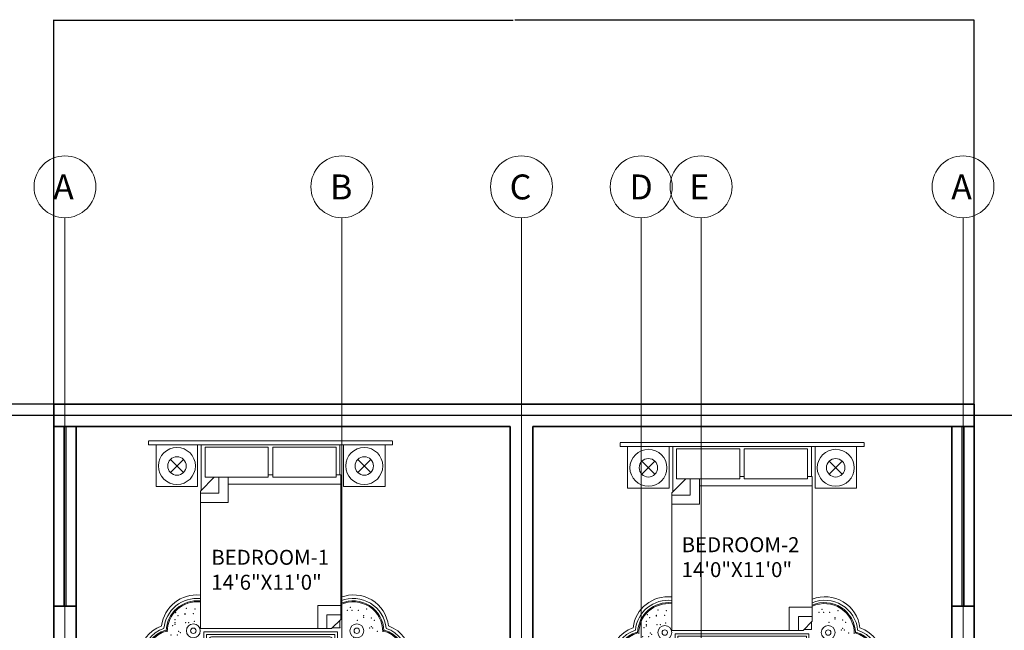
# Model space of a CAD drawing. Units: inches. Extents: x 5716 to 6907, y 12769 to 13594.
# Tile 16 of 17: x 6254 to 6648, y 13349 to 13594. Entities that reach past the tile are written whole.
import ezdxf

# ---------------------------------------------------------------- set-up
doc = ezdxf.new("R2010")
doc.units = ezdxf.units.IN
for name, color, linetype, lineweight in [('A-ANNO-DIMS', 2, 'Continuous', 18), ('A-AREA-IDEN', 7, 'Continuous', 18), ('A-FURN', 8, 'Continuous', 18), ('A-GLAZ', 4, 'Continuous', 18), ('A-GRID', 8, 'Continuous', 13), ('A-GRID-IDEN', 7, 'Continuous', 18), ('A-WALL', 7, 'Continuous', 35)]:
    doc.layers.add(name, color=color, linetype=linetype, lineweight=lineweight)
doc.styles.get("Standard").update_dxf_attribs({"font": 'arial.ttf'})
doc.dimstyles.get("Standard").update_dxf_attribs({"dimtxt": 0.18, "dimasz": 0.18, "dimexe": 0.18, "dimexo": 0.0625, "dimgap": 0.09, "dimtad": 0, "dimtih": 1, "dimtoh": 1, "dimdec": 4, "dimzin": 0, "dimdsep": 46, "dimtxsty": 'Standard', "dimcen": 0.09, "dimadec": 0, "dimazin": 0, "dimtfac": 1, "dimtdec": 4, "dimtofl": 0, "dimtmove": 0, "dimatfit": 3, "dimfxl": 1, "dimtolj": 1, "dimtzin": 0, "dimarcsym": 0})

# ---------------------------------------------------------------- blocks, each defined once
blk = doc.blocks.new('A$C1EC128A1')
for p, q in [((0.115, 3.56), (3.019, 3.56)), ((0.115, 3.555), (0.115, 3.511)), ((3.019, 3.555), (3.019, 3.511)), ((0.115, 3.511), (3.019, 3.511)), ((0.203, 3.511), (0.203, 3.462)), ((0.203, 3.46), (0.203, 3.016)), ((0.698, 3.511), (0.698, 3.016)), ((0.742, 3.511), (0.742, 2.972)), ((0.786, 3.484), (1.539, 3.484)), ((0.786, 3.484), (0.786, 3.126)), ((1.539, 3.126), (1.539, 3.484)), ((1.594, 3.126), (1.594, 3.484)), ((1.594, 3.484), (2.348, 3.484)), ((2.348, 3.484), (2.348, 3.126)), ((2.392, 3.511), (2.392, 3.154)), ((2.436, 3.511), (2.436, 3.016)), ((2.931, 3.511), (2.931, 3.016)), ((0.374, 3.181), (0.53, 3.337)), ((0.374, 3.337), (0.53, 3.181)), ((2.604, 3.337), (2.759, 3.181)), ((2.759, 3.337), (2.604, 3.181)), ((0.731, 2.961), (0.896, 3.126)), ((0.786, 3.126), (1.539, 3.126)), ((0.951, 3.126), (0.951, 2.934)), ((1.061, 3.126), (1.061, 2.824)), ((1.539, 3.154), (1.594, 3.154)), ((1.594, 3.126), (2.348, 3.126)), ((2.348, 3.154), (2.403, 3.154)), ((2.403, 3.154), (2.403, 1.432)), ((0.203, 3.016), (0.698, 3.016)), ((0.731, 2.961), (0.731, 1.322)), ((0.731, 2.934), (0.951, 2.934)), ((1.061, 3.044), (2.403, 3.044)), ((2.931, 3.016), (2.436, 3.016)), ((0.731, 2.824), (1.061, 2.824)), ((2.128, 1.597), (2.403, 1.597)), ((2.128, 1.597), (2.128, 1.322)), ((2.238, 1.487), (2.238, 1.322)), ((2.238, 1.487), (2.403, 1.487)), ((2.293, 1.322), (2.403, 1.432)), ((2.392, 1.421), (2.392, 1.333)), ((0.731, 1.322), (2.293, 1.322)), ((2.304, 1.333), (2.392, 1.333)), ((0.772, 1.282), (2.363, 1.282)), ((0.772, 0.939), (0.772, 1.282)), ((0.802, 1.252), (2.333, 1.252)), ((0.802, 0.969), (0.802, 1.252)), ((0.832, 1.029), (0.832, 1.192)), ((0.862, 1.222), (2.273, 1.222)), ((2.303, 1.192), (2.303, 1.029)), ((2.333, 1.252), (2.333, 0.969)), ((2.363, 1.282), (2.363, 0.939)), ((2.363, 0.939), (0.772, 0.939)), ((2.333, 0.969), (0.802, 0.969)), ((2.273, 0.999), (0.862, 0.999))]:
    blk.add_line(p, q)
for centre, radius in [((0.452, 3.259), 0.22), ((2.682, 3.259), 0.22), ((0.452, 3.259), 0.11), ((2.682, 3.259), 0.11), ((0.647, 1.296), 0.0826), ((0.647, 1.296), 0.0326), ((2.593, 1.296), 0.0826), ((2.593, 1.296), 0.0326), ((0.418, 0.972), 0.0826), ((0.418, 0.972), 0.0326), ((2.822, 0.972), 0.0826), ((2.822, 0.972), 0.0326), ((0.647, 0.647), 0.0826), ((2.593, 0.647), 0.0826), ((0.647, 0.647), 0.0326), ((2.593, 0.647), 0.0326), ((1.111, 0.374), 0.0826), ((1.111, 0.374), 0.0326), ((1.613, 0.323), 0.0826), ((1.613, 0.323), 0.0326), ((2.129, 0.374), 0.0826), ((2.129, 0.374), 0.0326)]:
    blk.add_circle(centre, radius)
for centre, radius, start, end in [((0.685, 1.305), 0.418, 83.7824, 173.2515), ((0.688, 1.288), 0.393, 83.8157, 174.53), ((0.692, 1.284), 0.369, 83.9971, 177.9976), ((2.555, 1.305), 0.418, 6.7485, 111.2795), ((2.552, 1.288), 0.393, 5.47, 112.249), ((2.548, 1.284), 0.369, 2.0024, 113.1536), ((0.691, 1.287), 0.354, 83.6051, 180.6699), ((2.549, 1.287), 0.354, 359.3301, 114.3551), ((0.405, 0.972), 0.405, 109.4527, 180), ((0.412, 0.972), 0.371, 108.0256, 180), ((0.411, 0.972), 0.343, 105.7891, 180), ((0.412, 0.972), 0.331, 104.766, 180), ((2.828, 0.972), 0.331, 0, 75.234), ((2.829, 0.972), 0.343, 0, 74.2109), ((2.828, 0.972), 0.371, 0, 71.9744), ((2.835, 0.972), 0.405, 0, 70.5473), ((0.862, 1.192), 0.03, 90, 180), ((2.273, 1.192), 0.03, 0, 90), ((2.008, 0.994), 0.365, 1.1782, 13.4812), ((0.405, 0.972), 0.405, 180, 250.5473), ((0.412, 0.972), 0.371, 180, 251.9744), ((0.411, 0.972), 0.343, 180, 254.2109), ((0.412, 0.972), 0.331, 180, 255.234), ((0.862, 1.029), 0.03, 180, 270), ((1.217, 0.977), 0.365, 186.0197, 214.7326), ((1.217, 0.977), 0.265, 188.3055, 214.7326), ((1.62, 0.972), 0.319, 185.9507, 354.0493), ((1.62, 0.972), 0.305, 186.2151, 353.7849), ((1.62, 0.972), 0.121, 195.7695, 344.2305), ((1.62, 0.972), 0.105, 198.3291, 341.6709), ((2.008, 0.994), 0.265, 327.6239, 348.1186), ((2.273, 1.029), 0.03, 270, 0), ((2.008, 0.994), 0.365, 327.6239, 1.1782), ((2.828, 0.972), 0.331, 284.766, 0), ((2.829, 0.972), 0.343, 285.7891, 0), ((2.828, 0.972), 0.371, 288.0256, 0), ((2.835, 0.972), 0.405, 289.4527, 0), ((1.403, 1.107), 0.492, 214.7326, 239.1926), ((1.817, 1.115), 0.492, 303.1639, 327.6239), ((1.403, 1.107), 0.592, 214.7326, 239.1926), ((1.817, 1.115), 0.592, 303.1639, 327.6239), ((0.685, 0.639), 0.418, 186.7485, 287.3233), ((0.688, 0.656), 0.393, 185.47, 288.0175), ((0.692, 0.66), 0.369, 182.0024, 288.623), ((0.691, 0.657), 0.354, 179.3301, 289.5945), ((1.524, 1.309), 0.828, 239.1926, 256.6746), ((1.524, 1.309), 0.728, 239.1926, 256.6746), ((1.599, 1.627), 1.054, 256.6746, 271.1782), ((1.599, 1.627), 1.054, 271.1782, 285.6819), ((1.688, 1.312), 0.728, 285.6819, 303.1639), ((1.688, 1.312), 0.828, 285.6819, 303.1639), ((2.549, 0.657), 0.354, 250.4055, 0.6699), ((2.548, 0.66), 0.369, 251.377, 357.9976), ((2.552, 0.656), 0.393, 251.9825, 354.53), ((2.555, 0.639), 0.418, 252.6767, 353.2515), ((1.599, 1.627), 1.154, 256.6746, 271.1782), ((1.599, 1.627), 1.154, 271.1782, 285.6819), ((1.133, 0.498), 0.367, 208.2914, 306.3479), ((1.133, 0.484), 0.367, 208.2914, 306.3479), ((1.133, 0.461), 0.369, 208.9302, 306.0262), ((1.132, 0.42), 0.369, 209.2201, 306.079), ((2.107, 0.498), 0.367, 233.6521, 331.7086), ((2.107, 0.484), 0.367, 233.6521, 331.7086), ((2.107, 0.461), 0.369, 233.9738, 331.0698), ((2.108, 0.42), 0.369, 233.921, 330.7799), ((1.614, 0.43), 0.349, 220.6393, 270.9052), ((1.614, 0.416), 0.349, 220.6393, 270.9052), ((1.62, 0.4), 0.36, 221.3878, 270), ((1.62, 0.36), 0.36, 221.4185, 270), ((1.626, 0.43), 0.349, 269.0948, 319.3607), ((1.626, 0.416), 0.349, 269.0948, 319.3607), ((1.62, 0.4), 0.36, 270, 318.6122), ((1.62, 0.36), 0.36, 270, 318.5815)]:
    blk.add_arc(centre, radius, start, end)
for p in [(0.565, 1.565), (0.666, 1.556), (2.482, 1.538), (2.518, 1.574), (2.537, 1.538), (2.61, 1.538), (2.71, 1.556), (0.428, 1.428), (0.438, 1.51), (0.465, 1.474), (0.547, 1.501), (0.547, 1.492), (0.647, 1.501), (0.657, 1.41), (2.601, 1.419), (2.674, 1.474), (2.674, 1.456), (2.765, 1.447), (2.801, 1.419), (0.401, 1.355), (0.428, 1.392), (0.428, 1.373), (0.474, 1.291), (0.556, 1.392), (0.593, 1.392), (2.392, 1.333), (2.747, 1.328), (2.765, 1.346), (2.783, 1.328), (2.838, 1.291), (0.319, 1.182), (0.383, 1.246), (0.456, 1.246), (0.474, 1.182), (0.492, 1.273), (0.556, 1.172), (2.555, 1.218), (0.118, 1.109), (0.182, 1.145), (0.209, 1.099), (0.237, 1.072), (0.246, 1.063), (0.301, 1.118), (0.456, 1.127), (0.657, 1.118), (2.455, 1.136), (2.482, 1.063), (2.646, 1.063), (2.774, 1.163), (2.893, 1.109), (2.966, 1.145), (3.057, 1.099), (0.118, 0.981), (0.155, 1.026), (0.182, 1.017), (0.182, 0.944), (0.593, 1.045), (0.684, 0.962), (1.303, 0.939), (1.317, 0.939), (2.473, 1.026), (2.537, 1.035), (2.573, 1.035), (2.601, 0.962), (2.966, 1.035), (0.173, 0.917), (0.182, 0.898), (0.209, 0.871), (0.474, 0.835), (0.602, 0.835), (0.666, 0.853), (0.693, 0.862), (0.812, 0.835), (0.999, 0.826), (1.067, 0.853), (1.076, 0.835), (1.113, 0.825), (1.186, 0.853), (1.259, 0.871), (1.277, 0.844), (2.026, 0.825), (2.044, 0.844), (2.044, 0.844), (2.153, 0.926), (2.153, 0.844), (2.591, 0.871), (2.984, 0.825), (3.002, 0.889), (3.002, 0.825), (3.102, 0.926), (0.173, 0.798), (0.255, 0.78), (0.264, 0.789), (0.301, 0.752), (0.511, 0.78), (0.784, 0.734), (0.803, 0.734), (1.067, 0.816), (1.113, 0.798), (1.159, 0.78), (1.159, 0.761), (1.204, 0.761), (1.25, 0.752), (1.259, 0.761), (1.259, 0.743), (1.259, 0.734), (1.277, 0.743), (1.305, 0.752), (1.314, 0.771), (1.323, 0.816), (1.898, 0.707), (1.907, 0.807), (1.907, 0.752), (2.062, 0.798), (2.381, 0.752), (2.409, 0.716), (2.418, 0.78), (2.537, 0.816), (2.591, 0.78), (2.756, 0.78), (2.829, 0.716), (2.847, 0.707), (2.883, 0.798), (0.31, 0.67), (0.401, 0.606), (0.41, 0.661), (0.447, 0.588), (0.465, 0.615), (0.492, 0.661), (0.821, 0.698), (0.903, 0.67), (0.912, 0.652), (0.949, 0.588), (1.152, 0.684), (1.152, 0.684), (1.152, 0.684), (1.286, 0.688), (1.323, 0.698), (1.323, 0.67), (1.35, 0.698), (1.35, 0.679), (1.356, 0.601), (1.359, 0.688), (1.451, 0.643), (1.487, 0.679), (1.578, 0.624), (1.651, 0.661), (1.651, 0.661), (1.779, 0.661), (1.88, 0.679), (1.88, 0.661), (1.884, 0.612), (2.007, 0.679), (2.086, 0.703), (2.263, 0.597), (2.381, 0.634), (2.4, 0.624), (2.737, 0.661), (0.465, 0.533), (0.501, 0.506), (0.529, 0.478), (0.593, 0.524), (0.73, 0.478), (0.73, 0.469), (0.757, 0.497), (0.812, 0.524), (0.83, 0.57), (0.867, 0.542), (0.967, 0.533), (0.976, 0.515), (1.031, 0.515), (1.333, 0.504), (1.898, 0.469), (2.19, 0.561), (2.263, 0.533), (2.272, 0.533), (2.409, 0.515), (2.455, 0.478), (2.482, 0.478), (2.61, 0.478), (2.646, 0.469), (2.747, 0.551), (2.756, 0.515), (2.81, 0.551), (0.465, 0.451), (0.538, 0.387), (0.556, 0.451), (0.574, 0.387), (0.602, 0.442), (0.62, 0.46), (0.638, 0.424), (0.739, 0.405), (0.739, 0.405), (0.912, 0.414), (0.921, 0.36), (0.93, 0.442), (0.985, 0.405), (1.341, 0.36), (1.396, 0.369), (1.414, 0.396), (1.642, 0.369), (1.77, 0.405), (1.852, 0.405), (2.144, 0.442), (2.245, 0.433), (2.29, 0.387), (2.601, 0.46), (0.638, 0.35), (0.693, 0.332), (0.81, 0.282), (0.985, 0.323), (1.086, 0.241), (1.204, 0.323), (1.213, 0.25), (1.332, 0.296), (1.341, 0.296), (1.35, 0.296), (1.378, 0.341), (1.496, 0.35), (1.651, 0.259), (1.852, 0.268), (1.87, 0.277), (1.916, 0.35), (2.327, 0.323), (2.43, 0.324), (0.985, 0.149), (1.131, 0.159), (1.35, 0.203), (1.451, 0.204), (1.487, 0.204), (1.606, 0.149), (1.67, 0.204), (1.724, 0.186), (1.962, 0.195), (2.08, 0.204), (2.135, 0.213), (2.217, 0.177)]:
    blk.add_point(p)
blk = doc.blocks.new('WIN-GLAZING-72IN')
for p, q in [((0, 0), (0, -72)), ((1, 0), (1, -72))]:
    blk.add_line(p, q)
blk = doc.blocks.new('*D49')
at = {"layer": 'A-ANNO-DIMS', "color": 0, "lineweight": -2, "transparency": 16777216}
for p, q in [((6267.41, 13440.21), (6267.41, 13594.38)), ((6267.59, 13594.2), (6451.62, 13594.2)), ((6636.23, 13594.2), (6452.2, 13594.2)), ((6636.41, 13440.21), (6636.41, 13594.38))]:
    blk.add_line(p, q, dxfattribs=at)
at = {"layer": 'A-ANNO-DIMS', "color": 0, "transparency": 16777216}
for points in [[(6267.59, 13594.23), (6267.59, 13594.17), (6267.41, 13594.2)], [(6636.23, 13594.23), (6636.23, 13594.17), (6636.41, 13594.2)]]:
    blk.add_solid(points, dxfattribs=at)
at = {"layer": 'Defpoints', "color": 0, "transparency": 16777216}
for p in [(6636.41, 13594.2), (6267.41, 13440.15), (6636.41, 13440.15)]:
    blk.add_point(p, dxfattribs=at)
at = {"layer": 'A-ANNO-DIMS', "color": 0, "transparency": 16777216, "insert": (6451.91, 13594.2), "char_height": 0.18, "attachment_point": 5}
blk.add_mtext('\\A1;369', dxfattribs=at)
blk = doc.blocks.new('*D52')
at = {"layer": 'A-ANNO-DIMS', "color": 0, "lineweight": -2, "transparency": 16777216}
for p, q in [((6267.34, 13440.15), (5716.04, 13440.15)), ((5716.22, 13439.97), (5716.22, 13140.83)), ((5716.22, 12841.33), (5716.22, 13140.47)), ((6267.34, 12841.15), (5716.04, 12841.15))]:
    blk.add_line(p, q, dxfattribs=at)
at = {"layer": 'A-ANNO-DIMS', "color": 0, "transparency": 16777216}
for points in [[(5716.19, 13439.97), (5716.25, 13439.97), (5716.22, 13440.15)], [(5716.19, 12841.33), (5716.25, 12841.33), (5716.22, 12841.15)]]:
    blk.add_solid(points, dxfattribs=at)
at = {"layer": 'Defpoints', "color": 0, "transparency": 16777216}
for p in [(6267.41, 13440.15), (5716.22, 12841.15), (6267.41, 12841.15)]:
    blk.add_point(p, dxfattribs=at)
at = {"layer": 'A-ANNO-DIMS', "color": 0, "transparency": 16777216, "insert": (5716.22, 13140.65), "char_height": 0.18, "attachment_point": 5}
blk.add_mtext('\\A1;599', dxfattribs=at)
blk = doc.blocks.new('*D58')
at = {"layer": 'A-ANNO-DIMS', "color": 0, "lineweight": -2, "transparency": 16777216}
for p, q in [((6736.67, 13435.65), (5716.04, 13435.65)), ((5716.22, 13435.47), (5716.22, 13365.33)), ((5716.22, 13294.83), (5716.22, 13364.97)), ((6736.67, 13294.65), (5716.04, 13294.65))]:
    blk.add_line(p, q, dxfattribs=at)
at = {"layer": 'A-ANNO-DIMS', "color": 0, "transparency": 16777216}
for points in [[(5716.19, 13435.47), (5716.25, 13435.47), (5716.22, 13435.65)], [(5716.19, 13294.83), (5716.25, 13294.83), (5716.22, 13294.65)]]:
    blk.add_solid(points, dxfattribs=at)
at = {"layer": 'Defpoints', "color": 0, "transparency": 16777216}
for p in [(6736.73, 13435.65), (5716.22, 13294.65), (6736.73, 13294.65)]:
    blk.add_point(p, dxfattribs=at)
at = {"layer": 'A-ANNO-DIMS', "color": 0, "transparency": 16777216, "insert": (5716.22, 13365.15), "char_height": 0.18, "attachment_point": 5}
blk.add_mtext('\\A1;141', dxfattribs=at)

msp = doc.modelspace()

# ---------------------------------------------------------------- linework, layer by layer
at = {"layer": 'A-GRID'}
for p, q in [((6271.91, 12841.15), (6271.91, 13514.96)), ((6382.91, 12841.15), (6382.91, 13514.96)), ((6454.91, 12841.15), (6454.91, 13514.96)), ((6502.91, 12841.15), (6502.91, 13514.96)), ((6526.91, 12841.15), (6526.91, 13514.96)), ((6631.91, 12841.15), (6631.91, 13514.96)), ((6267.41, 13435.65), (6736.73, 13435.65))]:
    msp.add_line(p, q, dxfattribs=at)
at = {"layer": 'A-GRID-IDEN'}
for centre in [(6271.91, 13527.35), (6382.91, 13527.35), (6454.91, 13527.35), (6502.91, 13527.35), (6526.91, 13527.35), (6631.91, 13527.35)]:
    msp.add_circle(centre, 12.4, dxfattribs=at)
at = {"layer": 'A-WALL'}
for p, q in [((6267.41, 13440.15), (6267.41, 12841.15)), ((6267.41, 13440.15), (6636.41, 13440.15)), ((6636.41, 13440.15), (6636.41, 13185.15)), ((6267.41, 13431.15), (6450.41, 13431.15)), ((6276.41, 13431.15), (6276.41, 13299.15)), ((6450.41, 13431.15), (6450.41, 13290.15)), ((6459.41, 13431.15), (6459.41, 13290.15)), ((6459.41, 13431.15), (6636.41, 13431.15)), ((6627.41, 13431.15), (6627.41, 13299.15)), ((6267.41, 13359.15), (6276.41, 13359.15)), ((6627.41, 13359.15), (6636.41, 13359.15))]:
    msp.add_line(p, q, dxfattribs=at)

# ---------------------------------------------------------------- block references
at = {"layer": 'A-FURN', "xscale": 33.66910864864256, "yscale": 33.66910864864256, "zscale": 33.66910864864256}
for p in [(6301.59, 13305.65), (6490.57, 13304.93)]:
    msp.add_blockref('A$C1EC128A1', p, dxfattribs=at)
at = {"layer": 'A-GLAZ', "rotation": 180}
for p in [(6272.41, 13359.15), (6632.41, 13359.15)]:
    msp.add_blockref('WIN-GLAZING-72IN', p, dxfattribs=at)

# ---------------------------------------------------------------- texts
at = {"layer": 'A-AREA-IDEN', "char_height": 6, "attachment_point": 1}
for s, width, insert in [('BEDROOM-2\\P14\'0"X11\'0"', 94.1172, (6519.12, 13386.81)), ('BEDROOM-1\\P14\'6"X11\'0"', 112.0121, (6330.58, 13381.75))]:
    msp.add_mtext_dynamic_manual_height_columns(s, width=width, gutter_width=12.5, heights=[0], dxfattribs=dict(at, insert=insert))
at = {"layer": 'A-GRID-IDEN', "char_height": 10, "attachment_point": 1}
for s, insert in [('A', (6267.17, 13532.29)), ('B', (6378.17, 13532.29)), ('C', (6450.17, 13532.29)), ('D', (6498.17, 13532.29)), ('E', (6522.17, 13532.29)), ('A', (6627.17, 13532.29))]:
    msp.add_mtext_dynamic_manual_height_columns(s, width=121.9272, gutter_width=12.5, heights=[0], dxfattribs=dict(at, insert=insert))

# ---------------------------------------------------------------- dimensions: what is measured, and where the dimension line sits
at = {"layer": 'A-ANNO-DIMS'}
dim = msp.add_linear_dim(base=(6636.41, 13594.2), p1=(6267.41, 13440.15), p2=(6636.41, 13440.15), dimstyle='Standard', override={"dimdec": 0, "dimlfac": 1, "dimrnd": 0, "dimzin": 0, "dimdsep": 46, "dimlunit": 2}, dxfattribs=at)
dim.commit()
dim.dimension.update_dxf_attribs({"geometry": '*D49', "text_midpoint": (6451.91, 13594.2)})
for base, p1, p2, picture, middle in [((5716.22, 12841.15), (6267.41, 13440.15), (6267.41, 12841.15), '*D52', (5716.22, 13140.65)), ((5716.22, 13294.65), (6736.73, 13435.65), (6736.73, 13294.65), '*D58', (5716.22, 13365.15))]:
    dim = msp.add_linear_dim(base=base, p1=p1, p2=p2, angle=90, dimstyle='Standard', override={"dimdec": 0, "dimlfac": 1, "dimrnd": 0, "dimzin": 0, "dimdsep": 46, "dimlunit": 2}, dxfattribs=at)
    dim.commit()
    dim.dimension.update_dxf_attribs({"geometry": picture, "text_midpoint": middle})

doc.saveas('drawing.dxf')
